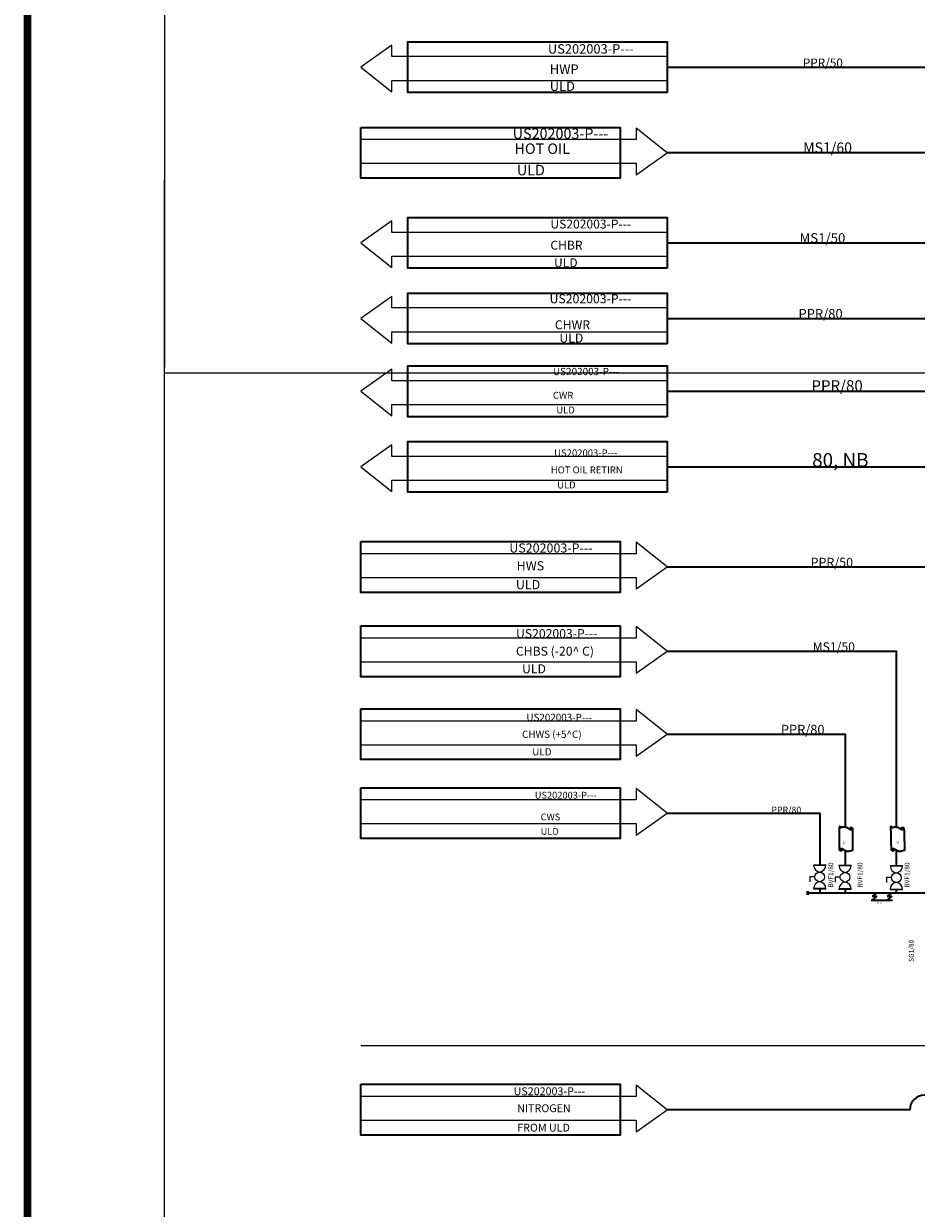
# Model space of a CAD drawing. Units: millimetres. Extents: x 353872 to 441597, y 126154 to 187356.
# Tile 3 of 28: x 353872 to 372047, y 143050 to 167178. Entities that reach past the tile are written whole.
import ezdxf

# ---------------------------------------------------------------- set-up
doc = ezdxf.new("R2010")
doc.units = ezdxf.units.MM
doc.linetypes.add('ACAD_ISO02W100', pattern=[15, 12, -3])
for name, color, linetype, lineweight in [('A-ANNO-DIMS', 2, 'Continuous', 18), ('P-ANNO-TEXT', 7, 'Continuous', 25), ('P-ANNO-TTLB', 7, 'Continuous', 25), ('P-BNDY', 4, 'ACAD_ISO02W100', 25), ('P-EQPM', 5, 'Continuous', 35), ('P-PIPE', 3, 'Continuous', 35), ('P-VALV', 2, 'Continuous', 25)]:
    doc.layers.add(name, color=color, linetype=linetype, lineweight=lineweight)
doc.styles.get("Standard").update_dxf_attribs({"font": 'arial.ttf'})
doc.dimstyles.get("Standard").update_dxf_attribs({"dimtxt": 0.18, "dimasz": 0.18, "dimexe": 0.18, "dimexo": 0.0625, "dimgap": 0.09, "dimtad": 0, "dimtih": 1, "dimtoh": 1, "dimdec": 4, "dimzin": 0, "dimdsep": 46, "dimtxsty": 'Standard', "dimcen": 0.09, "dimadec": 0, "dimazin": 0, "dimtfac": 1, "dimtdec": 4, "dimtofl": 0, "dimtmove": 0, "dimatfit": 3, "dimfxl": 1, "dimtolj": 1, "dimtzin": 0, "dimarcsym": 0})

# ---------------------------------------------------------------- blocks, each defined once
blk = doc.blocks.new('VALVE-A')
for points in [[(0, 9), (249, 9)], [(0, 6), (249, 6)], [(0, 3), (0, 0), (249, 0), (249, 4)], [(0, 3), (0, 3), (246, 3), (249, 3)]]:
    blk.add_lwpolyline(points)
for centre, radius, start, end in [((143, 1), 143, 97.3612, 180.5798), ((107, 2), 142, 359.2193, 82.8397)]:
    blk.add_arc(centre, radius, start, end)
blk = doc.blocks.new('VALVE-F')
for points in [[(0, 9), (249, 9)], [(0, 6), (249, 6)], [(0, 3), (0, 0), (249, 0), (249, 4)], [(0, 3), (0, 3), (246, 3), (249, 3)], [(124, 143), (124, 143)]]:
    blk.add_lwpolyline(points)
for centre, radius, start, end in [((143, 1), 143, 97.3612, 180.5798), ((107, 2), 142, 359.2193, 82.8397)]:
    blk.add_arc(centre, radius, start, end)
blk = doc.blocks.new('PIPE-FITTING-A')
blk.add_arc((29, 49), 33.1, 215.9005, 359.7553)
for points, weights, knots in [([(0, 23), (0, 175), (0, 328), (0, 481), (36, 493), (109, 520), (173, 476), (205, 454), (216, 447), (228, 445), (240, 449), (252, 453), (261, 462), (265, 473)], [1, 1, 1, 1, 1, 1, 1, 1, 0.930126763637, 0.930126763637, 1, 0.930126763637, 0.930126763637, 1], [0, 0, 0, 0, 1, 1, 1, 33.012448, 65.874064, 65.874064, 65.874064, 66.797942, 66.797942, 66.797942, 67.721819, 67.721819, 67.721819, 67.721819]), ([(205, 454), (205, 469), (214, 481), (228, 486), (242, 490), (257, 485), (265, 473), (266, 473), (266, 472), (267, 471), (267, 321), (267, 172), (267, 23), (231, 10), (158, -17), (94, 27), (62, 49), (51, 56), (39, 58), (27, 54), (15, 50), (6, 42), (2, 30)], [1, 0.872926124327, 0.872926124327, 1, 0.872926124327, 0.872926124327, 1, 1, 1, 1, 1, 1, 1, 1, 1, 1, 1, 0.930126763637, 0.930126763637, 1, 0.930126763637, 0.930126763637, 1], [0, 0, 0, 0, 1.25537, 1.25537, 1.25537, 2.51074, 2.51074, 2.51074, 3.51074, 3.51074, 3.51074, 4.51074, 4.51074, 4.51074, 36.523189, 69.384804, 69.384804, 69.384804, 70.308682, 70.308682, 70.308682, 71.232559, 71.232559, 71.232559, 71.232559])]:
    blk.add_rational_spline(points, weights, degree=3, knots=knots)
blk = doc.blocks.new('PIPE-FITTING-B')
for p, q in [((95, 147), (0, 84)), ((0, 84), (95, 84)), ((95, 84), (0, 0))]:
    blk.add_line(p, q)
blk = doc.blocks.new('*D25')
at = {"layer": 'A-ANNO-DIMS', "color": 0, "lineweight": -2, "transparency": 16777216}
for p, q in [((360736, 182546), (356736, 182546)), ((356737, 182546), (356737, 160180)), ((356737, 137813), (356737, 160179)), ((361696, 137813), (356736, 137813))]:
    blk.add_line(p, q, dxfattribs=at)
at = {"layer": 'A-ANNO-DIMS', "color": 0, "transparency": 16777216}
for points in [[(356737, 182546), (356737, 182546), (356737, 182546)], [(356737, 137813), (356737, 137813), (356737, 137813)]]:
    blk.add_solid(points, dxfattribs=at)
at = {"layer": 'Defpoints', "color": 0, "transparency": 16777216}
for p in [(360737, 182546), (356737, 137813), (361696, 137813)]:
    blk.add_point(p, dxfattribs=at)
at = {"layer": 'A-ANNO-DIMS', "color": 0, "transparency": 16777216, "insert": (356737, 160179), "char_height": 0.18, "attachment_point": 5}
blk.add_mtext('\\A1;44733', dxfattribs=at)
blk = doc.blocks.new('*D34')
at = {"layer": 'A-ANNO-DIMS', "color": 0, "lineweight": -2, "transparency": 16777216}
for p, q in [((399457, 167930), (356736, 167930)), ((356737, 167930), (356737, 163994)), ((356737, 160058), (356737, 163994)), ((399457, 160058), (356736, 160058))]:
    blk.add_line(p, q, dxfattribs=at)
at = {"layer": 'A-ANNO-DIMS', "color": 0, "transparency": 16777216}
for points in [[(356737, 167930), (356737, 167930), (356737, 167930)], [(356737, 160058), (356737, 160058), (356737, 160058)]]:
    blk.add_solid(points, dxfattribs=at)
at = {"layer": 'Defpoints', "color": 0, "transparency": 16777216}
for p in [(399457, 167930), (356737, 160058), (399457, 160058)]:
    blk.add_point(p, dxfattribs=at)
at = {"layer": 'A-ANNO-DIMS', "color": 0, "transparency": 16777216, "insert": (356737, 163994), "char_height": 0.18, "attachment_point": 5}
blk.add_mtext('\\A1;7872', dxfattribs=at)

msp = doc.modelspace()

# ---------------------------------------------------------------- linework, layer by layer
at = {"layer": 'P-ANNO-TTLB', "const_width": 152.43}
msp.add_lwpolyline([(353948.03, 187280.05), (353948.03, 126916.34), (440835.19, 126916.34), (440835.19, 187280.05)], close=True, dxfattribs=at)
at = {"layer": 'P-ANNO-TTLB'}
for points in [[(366976.76, 166506.67), (361369.95, 166506.67), (361369.95, 166740.65), (360736.55, 166292.58), (361369.95, 165789.54), (361369.95, 166023.52), (366976.76, 166023.52)], [(360736.55, 164334.83), (366343.35, 164334.83), (366343.35, 164100.85), (366976.76, 164548.92), (366343.35, 165051.96), (366343.35, 164817.98), (360736.55, 164817.98)], [(366976.76, 162927.96), (361369.95, 162927.96), (361369.95, 163161.94), (360736.55, 162713.87), (361369.95, 162210.82), (361369.95, 162444.81), (366976.76, 162444.81)], [(366976.76, 161387.94), (361369.95, 161387.94), (361369.95, 161621.92), (360736.55, 161173.85), (361369.95, 160670.81), (361369.95, 160904.79), (366976.76, 160904.79)], [(366976.76, 159905.17), (361369.95, 159905.17), (361369.95, 160139.15), (360736.55, 159691.08), (361369.95, 159188.04), (361369.95, 159422.02), (366976.76, 159422.02)], [(366976.76, 158365.16), (361369.95, 158365.16), (361369.95, 158599.14), (360736.55, 158151.07), (361369.95, 157648.02), (361369.95, 157882), (366976.76, 157882)], [(360736.55, 155898.89), (366343.35, 155898.89), (366343.35, 155664.91), (366976.76, 156112.98), (366343.35, 156616.03), (366343.35, 156382.05), (360736.55, 156382.05)], [(360736.55, 154181.75), (366343.35, 154181.75), (366343.35, 153947.77), (366976.76, 154395.83), (366343.35, 154898.88), (366343.35, 154664.9), (360736.55, 154664.9)], [(360736.55, 152492.29), (366343.35, 152492.29), (366343.35, 152258.31), (366976.76, 152706.38), (366343.35, 153209.43), (366343.35, 152975.45), (360736.55, 152975.45)], [(360736.55, 150885.93), (366343.35, 150885.93), (366343.35, 150651.95), (366976.76, 151100.02), (366343.35, 151603.07), (366343.35, 151369.09), (360736.55, 151369.09)], [(360736.55, 144844.56), (366343.35, 144844.56), (366343.35, 144610.57), (366976.76, 145058.64), (366343.35, 145561.69), (366343.35, 145327.71), (360736.55, 145327.71)]]:
    msp.add_lwpolyline(points, dxfattribs=at)
at = {"layer": 'P-BNDY'}
msp.add_line((360736.55, 146365.61), (391507.08, 146365.61), dxfattribs=at)
at = {"layer": 'P-EQPM'}
for points in [[(366976.76, 165774.97), (361695.78, 165774.97), (361695.78, 166810.19), (366976.76, 166810.19)], [(360736.55, 165066.53), (366017.52, 165066.53), (366017.52, 164031.31), (360736.55, 164031.31)], [(366976.76, 162196.26), (361695.78, 162196.26), (361695.78, 163231.48), (366976.76, 163231.48)], [(366976.76, 160656.24), (361695.78, 160656.24), (361695.78, 161691.47), (366976.76, 161691.47)], [(366976.76, 159173.47), (361695.78, 159173.47), (361695.78, 160208.69), (366976.76, 160208.69)], [(366976.76, 157633.45), (361695.78, 157633.45), (361695.78, 158668.68), (366976.76, 158668.68)], [(360736.55, 156630.59), (366017.52, 156630.59), (366017.52, 155595.37), (360736.55, 155595.37)], [(360736.55, 154913.45), (366017.52, 154913.45), (366017.52, 153878.22), (360736.55, 153878.22)], [(360736.55, 153223.99), (366017.52, 153223.99), (366017.52, 152188.77), (360736.55, 152188.77)], [(360736.55, 151617.63), (366017.52, 151617.63), (366017.52, 150582.41), (360736.55, 150582.41)], [(360736.55, 145576.26), (366017.52, 145576.26), (366017.52, 144541.03), (360736.55, 144541.03)]]:
    msp.add_lwpolyline(points, close=True, dxfattribs=at)
at = {"layer": 'P-PIPE'}
for p, q in [((369823.7, 149509.21), (369823.7, 149437.12)), ((369840.22, 149509.21), (369840.22, 149437.12)), ((369840.22, 149473.16), (374195.21, 149473.16)), ((370079.63, 149559.84), (370079.63, 149473.16)), ((370595.71, 149556.03), (370595.71, 149473.16)), ((371640.02, 149543.95), (371640.02, 149473.16)), ((371125.23, 149326.35), (371565.57, 149326.35))]:
    msp.add_line(p, q, dxfattribs=at)
for points in [[(366976.76, 166292.58), (378240.04, 166292.58), (378240.04, 150820.94)], [(366976.76, 162713.87), (368253.39, 162713.87)], [(368253.39, 162713.87), (377195.34, 162713.87), (377195.34, 150820.94)], [(366976.76, 161173.85), (376069.9, 161173.85), (376069.9, 150820.94)], [(366976.76, 159691.08), (375005.02, 159691.08), (375005.02, 150012.67)], [(366976.76, 158151.07), (373893.68, 158151.07), (373893.68, 150017.57)], [(366976.76, 156112.98), (372813.3, 156112.98), (372813.3, 150820.94)], [(366976.76, 154395.83), (371640.02, 154395.83), (371640.02, 150820.94)], [(366976.76, 152706.38), (370597.1, 152706.38), (370597.1, 150819.56)], [(366976.76, 151100.02), (370079.63, 151100.02), (370079.63, 150041.83)], [(370597.1, 150335.22), (370597.1, 150035.22)], [(371640.02, 150340.11), (371640.02, 150025.94)]]:
    msp.add_lwpolyline(points, dxfattribs=at)
for points in [[(380805, 150820.94), (380805, 164548.92), (380124.81, 164548.92, 1), (379436.2, 164548.92), (378584.35, 164548.92, 1), (377895.74, 164548.92), (366976.76, 164548.92)], [(383301.45, 145058.64, 1), (382877.96, 145058.64), (377035.77, 145058.64, 1), (376445.02, 145058.64), (372504.41, 145058.64, 1), (371913.66, 145058.64), (366976.76, 145058.64)]]:
    msp.add_lwpolyline(points, format="xyb", dxfattribs=at)
at = {"layer": 'P-VALV'}
for points in [[(369981.27, 149800.83), (369878.63, 149800.83), (369878.63, 149700.06)], [(370498.74, 149794.23), (370396.1, 149794.23), (370396.1, 149693.45)], [(371541.66, 149784.95), (371439.02, 149784.95), (371439.02, 149684.17)]]:
    msp.add_lwpolyline(points, dxfattribs=at)
for centre in [(370079.3, 149800.83), (370596.77, 149794.23), (371639.69, 149784.95)]:
    msp.add_circle(centre, 98.03, dxfattribs=at)

# ---------------------------------------------------------------- block references
at = {"layer": 'P-PIPE'}
for name, p in [('PIPE-FITTING-A', (370483.66, 150318.51)), ('PIPE-FITTING-B', (371145.99, 149326.35)), ('PIPE-FITTING-B', (371454.76, 149326.35))]:
    msp.add_blockref(name, p, dxfattribs=at)
at = {"layer": 'P-PIPE', "rotation": 1.588978313683039}
msp.add_blockref('PIPE-FITTING-A', (371542.17, 150314.09), dxfattribs=at)
at = {"layer": 'P-VALV'}
for name, p, rotation in [('VALVE-F', (370203.21, 150044.54), 181.2525321959233), ('VALVE-A', (370720.93, 150038.04), 181.3019170020234), ('VALVE-A', (371763.85, 150028.76), 181.3019170020368)]:
    msp.add_blockref(name, p, dxfattribs=dict(at, rotation=rotation))
for name, p in [('VALVE-F', (369955.26, 149559.84)), ('VALVE-A', (370472.73, 149553.23)), ('VALVE-A', (371515.65, 149543.95))]:
    msp.add_blockref(name, p, dxfattribs=at)

# ---------------------------------------------------------------- texts
at = {"layer": 'P-ANNO-TEXT'}
for s, height, p in [('US202003-P---', 191.8516, (364546.6, 166567.98)), ('PPR/50', 175.569, (369736.32, 166292.58)), ('HWP', 191.852, (364585.08, 166156.04)), ('ULD', 191.852, (364583.96, 165806.91)), ('US202003-P---', 214.3034, (363828.38, 164832.15)), ('HOT OIL', 214.303, (363864.52, 164525.01)), ('MS1/60', 210.227, (369743.66, 164548.92)), ('ULD', 214.303, (363914.27, 164089.42)), ('US202003-P---', 180.4668, (364596.35, 163006.6)), ('MS1/50', 197.144, (369670.16, 162713.87)), ('CHBR', 180.467, (364596.35, 162576.35)), ('ULD', 180.467, (364670.39, 162219.82)), ('US202003-P---', 183.0061, (364579.93, 161483.88)), ('PPR/80', 193.76, (369648.13, 161173.85)), ('CHWR', 183.006, (364686.57, 160954)), ('ULD', 183.006, (364779.39, 160684.37)), ('US202003-P---', 148.6139, (364647.79, 160019.41)), ('PPR/80', 225.254, (369910.81, 159691.08)), ('CWR', 141.612, (364647.79, 159538.42)), ('ULD', 141.612, (364716.79, 159239.3)), ('US202003-P---', 141.6119, (364673.91, 158365.16)), ('80, NB', 281.196, (369926.97, 158151.07)), ('HOT OIL RETIRN', 141.6119, (364605.87, 158018.17)), ('ULD', 141.612, (364733.86, 157711.21)), ('US202003-P---', 186.1677, (363760.05, 156406.31)), ('HWS', 186.168, (363909.24, 156043.84)), ('PPR/50', 186.168, (369895.03, 156112.98)), ('ULD', 186.168, (363894.16, 155659.97)), ('US202003-P---', 182.1693, (363896.18, 154664.9)), ('CHBS (-20^  C)', 182.1693, (363894.8, 154306.04)), ('MS1/50', 182.169, (369936.65, 154395.83)), ('ULD', 182.169, (364019.75, 153947.76)), ('US202003-P---', 147.0465, (364107.94, 152975.45)), ('CHWS (+5^ C)', 147.0465, (364019.13, 152631.57)), ('PPR/80', 191.312, (369289.56, 152706.38)), ('ULD', 147.046, (364227.1, 152274.85)), ('US202003-P---', 138.5753, (364277.64, 151395.06)), ('CWS', 138.575, (364397.61, 150952.84)), ('PPR/80', 130.771, (369096.86, 151100.02)), ('ULD', 138.575, (364397.61, 150657.2)), ('1HC', 39.332, (371240.04, 149254.36)), ('US202003-P---', 159.8074, (363848.19, 145354.22)), ('NITROGEN', 159.807, (363921.32, 145008.31)), ('FROM ULD', 159.807, (363921.32, 144612.69))]:
    msp.add_text(s, height=height, dxfattribs=at).set_placement(p)
for s, height, p in [('IC', 46.014, (370599.79, 150471.74)), ('IC', 46.014, (371691.01, 150471.74)), ('BVF1/80', 98.09, (370356.15, 149580.58)), ('BVF1/80', 98.09, (370950.08, 149580.58)), ('BVF1/80', 98.09, (371907.19, 149580.58)), ('SG1/80', 98.09, (371992.73, 148070.97))]:
    msp.add_text(s, height=height, rotation=90, dxfattribs=at).set_placement(p)

# ---------------------------------------------------------------- dimensions: what is measured, and where the dimension line sits
at = {"layer": 'A-ANNO-DIMS'}
for base, p1, p2, picture, middle in [((356736.55, 137812.84), (360736.55, 182546.05), (361695.78, 137812.84), '*D25', (356736.55, 160179.44)), ((356736.55, 160058.19), (399457.15, 167929.97), (399457.15, 160058.19), '*D34', (356736.55, 163994.08))]:
    dim = msp.add_linear_dim(base=base, p1=p1, p2=p2, angle=90, dimstyle='Standard', override={"dimdec": 0, "dimlfac": 1, "dimrnd": 0, "dimzin": 0, "dimdsep": 46, "dimlunit": 2}, dxfattribs=at)
    dim.commit()
    dim.dimension.update_dxf_attribs({"geometry": picture, "text_midpoint": middle})

doc.saveas('drawing.dxf')
